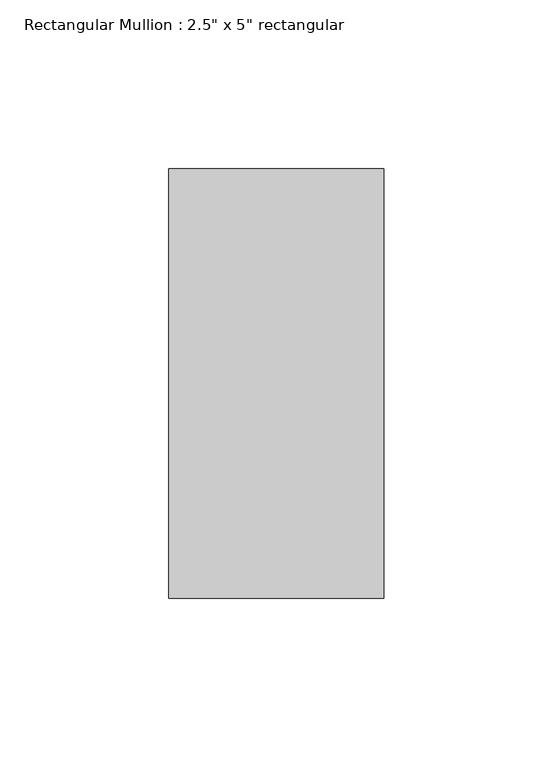
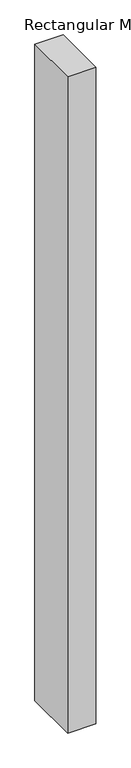
"""IFC4 building model written with IfcOpenShell, lengths in millimetres: member geometry."""

from ifc_helpers import new_model, si_unit, frame, origin, place, context, project, spatial, polyline, outline, extrude, source, transform, mapped, element, save


def member_7f03512f(model_context):
    return source(origin(), model_context, "Body", "SweptSolid", [
        extrude(outline(polyline([(0.0, 63.5), (0.0, -63.5), (-63.5, -63.5), (-63.5, 63.5), (0.0, 63.5)])), frame((0.0, 0.0, -1558.73195), z_axis=(0.0, 0.0, 1.0), x_axis=(1.0, 0.0, 0.0)), (0.0, 0.0, 1.0), 1558.73195),
    ])


if __name__ == "__main__":
    model = new_model("IFC4")
    model_context = context("Model", 3, world=origin())
    ifc_project = project(units=[si_unit("LENGTHUNIT", "METRE", prefix="MILLI")], contexts=[model_context])
    site = spatial("IfcSite", under=ifc_project)
    building = spatial("IfcBuilding", under=site)
    placement = place(None, origin())
    member_shape = member_7f03512f(model_context)
    element("IfcMember", 1, ObjectType="Rectangular Mullion : 2.5\" x 5\" rectangular", at=placement, inside=building, context=model_context, shape_type="MappedRepresentation", body=[
        mapped(member_shape, transform((0.0, 0.0, 0.0), x_axis=(1.0, 0.0, 0.0), y_axis=(0.0, 1.0, 0.0), z_axis=(0.0, 0.0, 1.0))),
    ])
    save(model, "model.ifc")

# Revit data of these elements
# Type "Rectangular Mullion : 2.5\" x 5\" rectangular"
#   built-in parameter 1007304 = 0.416667 (stored number, unit not read)
#   built-in parameter 1007301 = 0.104167 (stored number, unit not read)
#   built-in parameter 1007300 = 0.104167 (stored number, unit not read)
# Element 1 (IfcMember, "Rectangular Mullion : 2.5\" x 5\" rectangular")
#   Materials on its faces: "Aluminum"
# Materials
#   "Aluminum": class "Metal", colour RGB 247 247 247, transparency 0, Description = "Aluminum 6061", Cost = 0
